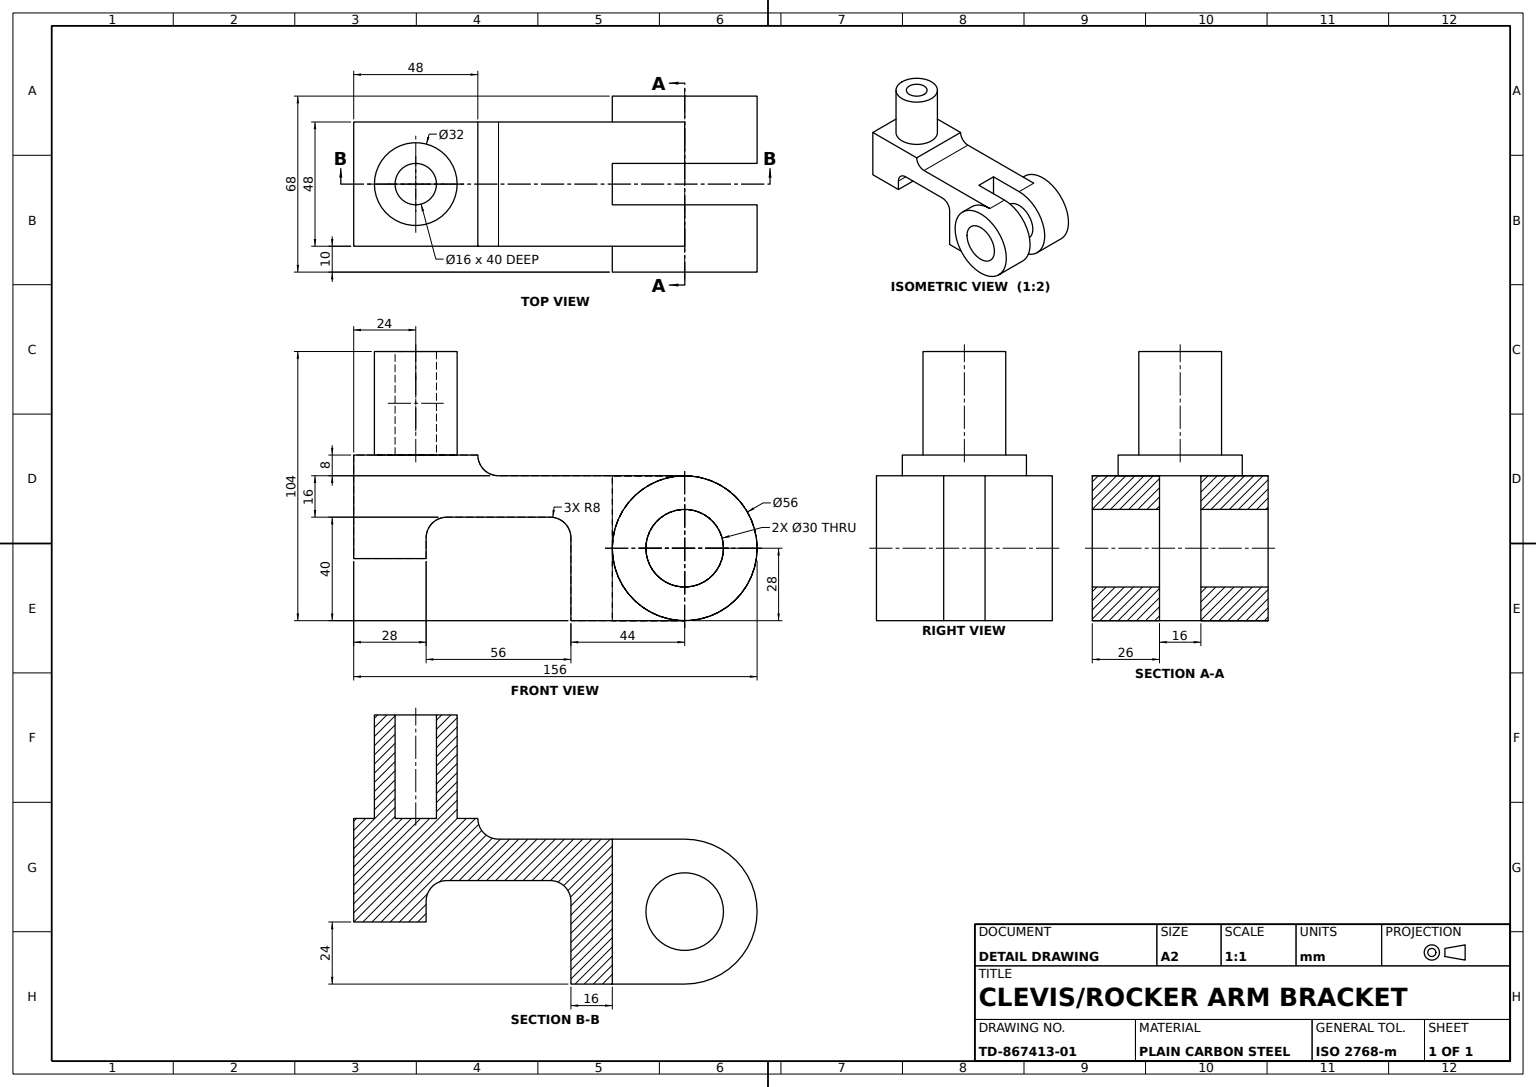
SolidWorks part; units mm, degrees
material "Plain Carbon Steel"
ref_plane "Front Plane" through (0, 0, 0) normal (0, 0, 1) x (1, 0, 0)
ref_plane "Top Plane" through (0, 0, 0) normal (0, 1, 0) x (1, 0, 0)
ref_plane "Right Plane" through (0, 0, 0) normal (1, 0, 0) x (0, 0, -1)
sketch "Arm Profile Sketch" plane through (0, 0, 0) normal (0, 0, 1) x (1, 0, 0)
  line L0 (0, 0) -> (28, 0)
  line L1 (28, 0) -> (28, 8)
  line L2 (36, 16) -> (76, 16)
  line L3 (84, 8) -> (84, -24)
  line L4 (84, -24) -> (128, -24)
  line L5 (128, -24) -> (128, 32)
  line L6 (128, 32) -> (56, 32)
  line L7 (48, 40) -> (0, 40)
  line L8 (0, 40) -> (0, 0)
  arc A0 (56, 32) -> (48, 40) centre (56, 40) cw
  arc A1 (76, 16) -> (84, 8) centre (76, 8) cw
  arc A2 (28, 8) -> (36, 16) centre (36, 8) cw
  point P14 (84, 16)
  point P17 (28, 16)
  dimension "D4" = 8
  dimension "D10" = 8
  dimension "D1" = 28
  dimension "D2" = 40
  dimension "D3" = 48
  dimension "D5" = 72
  dimension "D6" = 16
  dimension "D7" = 56
  dimension "D8" = 40
  dimension "D9" = 56
extrude "Arm Body" add sketch "Arm Profile Sketch" along normal mid plane 48
sketch "Bushing Boss Sketch" plane through (0, 40, 0) normal (0, 1, 0) x (1, 0, 0)
  circle A0 centre (24, 0) radius 16
  circle A1 centre (24, 0) radius 8
  dimension "D1" = 16
  dimension "D2" = 32
  dimension "D3" = 24
extrude "Bushing Boss Ø32" add sketch "Bushing Boss Sketch" along normal blind 40
sketch "Pivot Lug Sketch" plane through (0, 0, 0) normal (0, 0, 1) x (1, 0, 0)
  line L0 (128, -24) -> (128, 32) construction
  line L1 (128, 32) -> (56, 32) construction
  circle A1 centre (128, 4) radius 28
  dimension "D2" = 56
extrude "Pivot Lug Ø56" add sketch "Pivot Lug Sketch" along normal mid plane 68
sketch "Clevis Slot Sketch" plane through (0, 32, 0) normal (0, 1, 0) x (1, 0, 0)
  line L0 (100, -8) -> (100, 8)
  line L1 (100, -8) -> (156, -8)
  line L2 (100, 8) -> (156, 8)
  line L3 (156, -8) -> (156, 8)
  line L4 (128, -24) -> (128, 24) construction
  point P0 (100, 0)
  dimension "D1" = 16
  dimension "D2" = 28
  dimension "D3" = 56
extrude "Clevis Slot 16mm" cut sketch "Clevis Slot Sketch" against normal through all
hole_wizard "Pivot Bore Ø30" positions "Sketch7" profile "Sketch8" hole size "Ø1.0" standard "ANSI Metric" end condition through all
sketch "Sketch7" plane through (0, 0, 34) normal (0, 0, 1) x (1, 0, 0)
  point P0 (128, 4)
sketch "Sketch8" plane through (128, 4, 34) normal (1, 0, 0) x (0, -1, 0)
  line L0 (0, 0) -> (0, 68)
  line L1 (0, 68) -> (15, 68)
  line L2 (15, 68) -> (15, 0)
  line L5 (15, 0) -> (0, 0)
  line L11 (0, -6.35) -> (0, 107.95) construction
  dimension "Thru Hole Dia." = 30
  dimension "Thru Hole Depth" = 68
